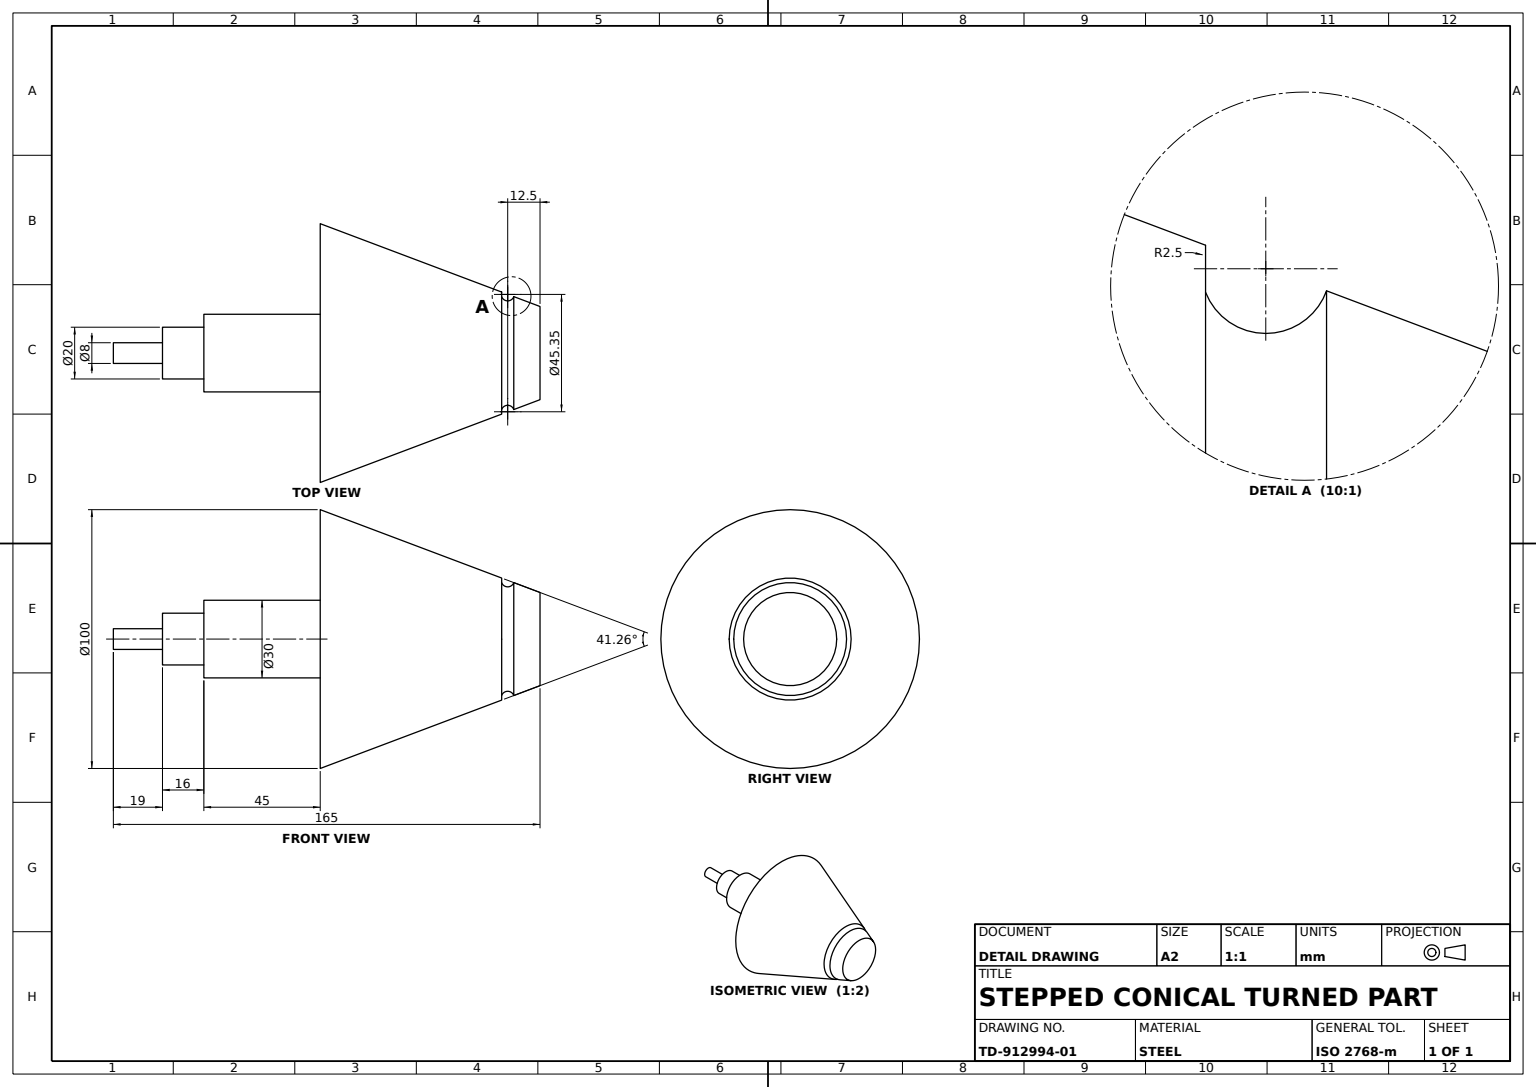
SolidWorks part; units mm, degrees
material "Plain Carbon Steel"
ref_plane "Front Plane" through (0, 0, 0) normal (0, 0, 1) x (1, 0, 0)
ref_plane "Top Plane" through (0, 0, 0) normal (0, 1, 0) x (1, 0, 0)
ref_plane "Right Plane" through (0, 0, 0) normal (1, 0, 0) x (0, 0, -1)
sketch "Shaft Base Ø30 Sketch" plane through (0, 0, 0) normal (0, 0, 1) x (1, 0, 0)
  circle A0 centre (0, 0) radius 15
  dimension "D1" = 30
extrude "Shaft Base Ø30" add sketch "Shaft Base Ø30 Sketch" along normal blind 45
sketch "Shaft Step 2 Sketch" plane through (0, 0, 45) normal (0, 0, 1) x (1, 0, 0)
  circle A0 centre (0, 0) radius 10
  dimension "D1" = 20
extrude "Shaft Step 2" add sketch "Shaft Step 2 Sketch" along normal blind 16
sketch "Shaft Tip Sketch" plane through (0, 0, 61) normal (0, 0, 1) x (1, 0, 0)
  circle A0 centre (0, 0) radius 4
  dimension "D1" = 8
extrude "Shaft Tip" add sketch "Shaft Tip Sketch" along normal blind 19
sketch "Cone Base Ø100 Sketch" plane through (0, 0, 0) normal (0, 0, -1) x (-1, 0, 0)
  circle A0 centre (0, 0) radius 50
  dimension "50" = 100
ref_plane "Cone Small End Plane" through (0, 0, -85) normal (0, 0, -1) x (-1, 0, 0)
sketch "Cone Small End Ø36 Sketch" plane through (0, 0, -85) normal (0, 0, -1) x (-1, 0, 0)
  circle A0 centre (0, 0) radius 18
  dimension "D1" = 36
loft "Conical Body" add profiles "Cone Small End Ø36 Sketch", "Cone Base Ø100 Sketch"
ref_plane "Groove Plane" through (0, 0, -72.5) normal (0, 0, -1) x (-1, 0, 0)
sketch "Groove Path" plane through (0, 0, -72.5) normal (0, 0, -1) x (-1, 0, 0)
  circle A0 centre (0, 0) radius 22.6735
  dimension "D1" = 45.3469
sweep "Groove Sweep Cut" cut path "Groove Path" circular profile diameter 5 parameters "D3"=5
